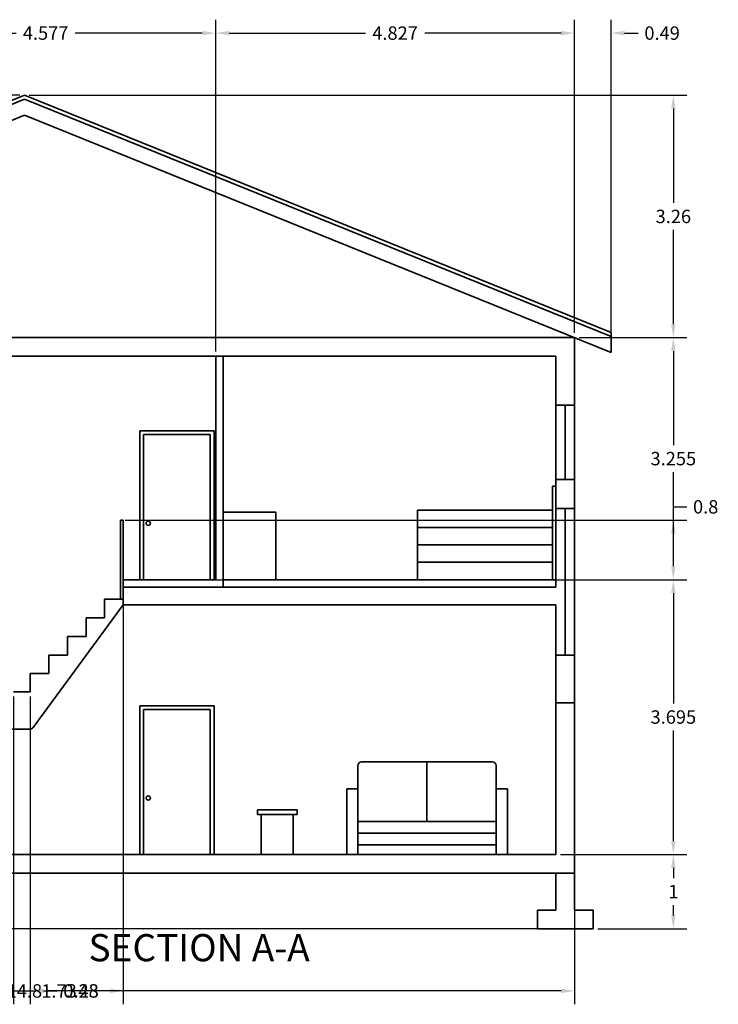
# Model space of a CAD drawing. Units: metres. Extents: x 14054 to 28215, y 4175 to 8383.
# Tile 6 of 6: x 14106.56 to 14115.96, y 4179.48 to 4192.72. Entities that reach past the tile are written whole.
import ezdxf

# ---------------------------------------------------------------- set-up
doc = ezdxf.new("R2010")
doc.units = ezdxf.units.M
for name, color, linetype, lineweight in [('A-ANNO-DIMS', 2, 'Continuous', 18), ('A-ANNO-NPLT', 9, 'Continuous', 13), ('A-ANNO-TEXT', 3, 'Continuous', 18), ('A-SECT', 1, 'Continuous', 35)]:
    doc.layers.add(name, color=color, linetype=linetype, lineweight=lineweight)
doc.styles.get("Standard").update_dxf_attribs({"font": 'arial.ttf'})
doc.dimstyles.get("Standard").update_dxf_attribs({"dimtxt": 0.18, "dimasz": 0.18, "dimexe": 0.18, "dimexo": 0.0625, "dimgap": 0.09, "dimtad": 0, "dimtih": 1, "dimtoh": 1, "dimdec": 4, "dimzin": 0, "dimdsep": 46, "dimtxsty": 'Standard', "dimcen": 0.09, "dimadec": 0, "dimazin": 0, "dimtfac": 1, "dimtdec": 4, "dimtofl": 0, "dimtmove": 0, "dimatfit": 3, "dimfxl": 1, "dimtolj": 1, "dimtzin": 0, "dimarcsym": 0})

# ---------------------------------------------------------------- blocks, each defined once
blk = doc.blocks.new('*D31')
at = {"layer": 'A-ANNO-DIMS', "color": 0, "lineweight": -2, "transparency": 16777216}
for p, q in [((14104.618, 4188.257), (14104.618, 4192.719)), ((14109.195, 4188.257), (14109.195, 4192.719)), ((14104.798, 4192.539), (14106.509, 4192.539)), ((14109.015, 4192.539), (14107.304, 4192.539))]:
    blk.add_line(p, q, dxfattribs=at)
at = {"layer": 'A-ANNO-DIMS', "color": 0, "transparency": 16777216}
for points in [[(14104.798, 4192.569), (14104.798, 4192.509), (14104.618, 4192.539)], [(14109.015, 4192.569), (14109.015, 4192.509), (14109.195, 4192.539)]]:
    blk.add_solid(points, dxfattribs=at)
at = {"layer": 'Defpoints', "color": 0, "transparency": 16777216}
for p in [(14109.195, 4192.539), (14104.618, 4188.194), (14109.195, 4188.194)]:
    blk.add_point(p, dxfattribs=at)
at = {"layer": 'A-ANNO-DIMS', "color": 0, "transparency": 16777216, "insert": (14106.907, 4192.539), "char_height": 0.18, "attachment_point": 5}
blk.add_mtext('\\A1;4.577', dxfattribs=at)
blk = doc.blocks.new('*D32')
at = {"layer": 'A-ANNO-DIMS', "color": 0, "lineweight": -2, "transparency": 16777216}
for p, q in [((14109.195, 4188.257), (14109.195, 4192.719)), ((14114.022, 4188.507), (14114.022, 4192.719)), ((14109.375, 4192.539), (14111.211, 4192.539)), ((14113.842, 4192.539), (14112.006, 4192.539))]:
    blk.add_line(p, q, dxfattribs=at)
at = {"layer": 'A-ANNO-DIMS', "color": 0, "transparency": 16777216}
for points in [[(14109.375, 4192.569), (14109.375, 4192.509), (14109.195, 4192.539)], [(14113.842, 4192.569), (14113.842, 4192.509), (14114.022, 4192.539)]]:
    blk.add_solid(points, dxfattribs=at)
at = {"layer": 'Defpoints', "color": 0, "transparency": 16777216}
for p in [(14114.022, 4192.539), (14114.022, 4188.444), (14109.195, 4188.194)]:
    blk.add_point(p, dxfattribs=at)
at = {"layer": 'A-ANNO-DIMS', "color": 0, "transparency": 16777216, "insert": (14111.608, 4192.539), "char_height": 0.18, "attachment_point": 5}
blk.add_mtext('\\A1;4.827', dxfattribs=at)
blk = doc.blocks.new('*D33')
at = {"layer": 'A-ANNO-DIMS', "color": 0, "lineweight": -2, "transparency": 16777216}
for p, q in [((14114.022, 4188.507), (14114.022, 4192.719)), ((14114.516, 4188.307), (14114.516, 4192.719)), ((14113.842, 4192.539), (14113.662, 4192.539)), ((14114.696, 4192.539), (14114.876, 4192.539))]:
    blk.add_line(p, q, dxfattribs=at)
at = {"layer": 'A-ANNO-DIMS', "color": 0, "transparency": 16777216}
for points in [[(14113.842, 4192.569), (14113.842, 4192.509), (14114.022, 4192.539)], [(14114.696, 4192.569), (14114.696, 4192.509), (14114.516, 4192.539)]]:
    blk.add_solid(points, dxfattribs=at)
at = {"layer": 'Defpoints', "color": 0, "transparency": 16777216}
for p in [(14114.516, 4192.539), (14114.022, 4188.444), (14114.516, 4188.244)]:
    blk.add_point(p, dxfattribs=at)
at = {"layer": 'A-ANNO-DIMS', "color": 0, "transparency": 16777216, "insert": (14115.2, 4192.539), "char_height": 0.18, "attachment_point": 5}
blk.add_mtext('\\A1;0.49', dxfattribs=at)
blk = doc.blocks.new('*D34')
at = {"layer": 'A-ANNO-DIMS', "color": 0, "lineweight": -2, "transparency": 16777216}
for p, q in [((14099.222, 4181.182), (14099.222, 4179.479)), ((14114.022, 4181.182), (14114.022, 4179.479)), ((14099.402, 4179.659), (14106.306, 4179.659)), ((14113.842, 4179.659), (14106.937, 4179.659))]:
    blk.add_line(p, q, dxfattribs=at)
at = {"layer": 'A-ANNO-DIMS', "color": 0, "transparency": 16777216}
for points in [[(14099.402, 4179.689), (14099.402, 4179.629), (14099.222, 4179.659)], [(14113.842, 4179.689), (14113.842, 4179.629), (14114.022, 4179.659)]]:
    blk.add_solid(points, dxfattribs=at)
at = {"layer": 'Defpoints', "color": 0, "transparency": 16777216}
for p in [(14099.222, 4181.244), (14114.022, 4181.244), (14114.022, 4179.659)]:
    blk.add_point(p, dxfattribs=at)
at = {"layer": 'A-ANNO-DIMS', "color": 0, "transparency": 16777216, "insert": (14106.622, 4179.659), "char_height": 0.18, "attachment_point": 5}
blk.add_mtext('\\A1;14.8', dxfattribs=at)
blk = doc.blocks.new('*D35')
at = {"layer": 'A-ANNO-DIMS', "color": 0, "lineweight": -2, "transparency": 16777216}
for p, q in [((14113.834, 4181.494), (14115.531, 4181.494)), ((14115.351, 4181.314), (14115.351, 4181.174)), ((14115.351, 4180.674), (14115.351, 4180.814)), ((14114.334, 4180.494), (14115.531, 4180.494))]:
    blk.add_line(p, q, dxfattribs=at)
at = {"layer": 'A-ANNO-DIMS', "color": 0, "transparency": 16777216}
for points in [[(14115.321, 4181.314), (14115.381, 4181.314), (14115.351, 4181.494)], [(14115.321, 4180.674), (14115.381, 4180.674), (14115.351, 4180.494)]]:
    blk.add_solid(points, dxfattribs=at)
at = {"layer": 'Defpoints', "color": 0, "transparency": 16777216}
for p in [(14113.772, 4181.494), (14115.351, 4181.494), (14114.272, 4180.494)]:
    blk.add_point(p, dxfattribs=at)
at = {"layer": 'A-ANNO-DIMS', "color": 0, "transparency": 16777216, "insert": (14115.351, 4180.994), "char_height": 0.18, "attachment_point": 5}
blk.add_mtext('\\A1;1', dxfattribs=at)
blk = doc.blocks.new('*D36')
at = {"layer": 'A-ANNO-DIMS', "color": 0, "lineweight": -2, "transparency": 16777216}
for p, q in [((14113.834, 4185.189), (14115.531, 4185.189)), ((14115.351, 4185.009), (14115.351, 4183.524)), ((14115.351, 4181.674), (14115.351, 4183.16)), ((14113.834, 4181.494), (14115.531, 4181.494))]:
    blk.add_line(p, q, dxfattribs=at)
at = {"layer": 'A-ANNO-DIMS', "color": 0, "transparency": 16777216}
for points in [[(14115.321, 4185.009), (14115.381, 4185.009), (14115.351, 4185.189)], [(14115.321, 4181.674), (14115.381, 4181.674), (14115.351, 4181.494)]]:
    blk.add_solid(points, dxfattribs=at)
at = {"layer": 'Defpoints', "color": 0, "transparency": 16777216}
for p in [(14113.772, 4185.189), (14115.351, 4185.189), (14113.772, 4181.494)]:
    blk.add_point(p, dxfattribs=at)
at = {"layer": 'A-ANNO-DIMS', "color": 0, "transparency": 16777216, "insert": (14115.351, 4183.342), "char_height": 0.18, "attachment_point": 5}
blk.add_mtext('\\A1;3.695', dxfattribs=at)
blk = doc.blocks.new('*D37')
at = {"layer": 'A-ANNO-DIMS', "color": 0, "lineweight": -2, "transparency": 16777216}
for p, q in [((14114.084, 4188.444), (14115.531, 4188.444)), ((14115.351, 4188.264), (14115.351, 4186.999)), ((14115.351, 4185.369), (14115.351, 4186.635)), ((14113.834, 4185.189), (14115.531, 4185.189))]:
    blk.add_line(p, q, dxfattribs=at)
at = {"layer": 'A-ANNO-DIMS', "color": 0, "transparency": 16777216}
for points in [[(14115.321, 4188.264), (14115.381, 4188.264), (14115.351, 4188.444)], [(14115.321, 4185.369), (14115.381, 4185.369), (14115.351, 4185.189)]]:
    blk.add_solid(points, dxfattribs=at)
at = {"layer": 'Defpoints', "color": 0, "transparency": 16777216}
for p in [(14114.022, 4188.444), (14115.351, 4188.444), (14113.772, 4185.189)]:
    blk.add_point(p, dxfattribs=at)
at = {"layer": 'A-ANNO-DIMS', "color": 0, "transparency": 16777216, "insert": (14115.351, 4186.817), "char_height": 0.18, "attachment_point": 5}
blk.add_mtext('\\A1;3.255', dxfattribs=at)
blk = doc.blocks.new('*D38')
at = {"layer": 'A-ANNO-DIMS', "color": 0, "lineweight": -2, "transparency": 16777216}
for p, q in [((14106.684, 4191.704), (14115.531, 4191.704)), ((14115.351, 4191.524), (14115.351, 4190.256)), ((14115.351, 4188.624), (14115.351, 4189.892)), ((14114.084, 4188.444), (14115.531, 4188.444))]:
    blk.add_line(p, q, dxfattribs=at)
at = {"layer": 'A-ANNO-DIMS', "color": 0, "transparency": 16777216}
for points in [[(14115.321, 4191.524), (14115.381, 4191.524), (14115.351, 4191.704)], [(14115.321, 4188.624), (14115.381, 4188.624), (14115.351, 4188.444)]]:
    blk.add_solid(points, dxfattribs=at)
at = {"layer": 'Defpoints', "color": 0, "transparency": 16777216}
for p in [(14106.622, 4191.704), (14115.351, 4191.704), (14114.022, 4188.444)]:
    blk.add_point(p, dxfattribs=at)
at = {"layer": 'A-ANNO-DIMS', "color": 0, "transparency": 16777216, "insert": (14115.351, 4190.074), "char_height": 0.18, "attachment_point": 5}
blk.add_mtext('\\A1;3.26', dxfattribs=at)
blk = doc.blocks.new('*D39')
at = {"layer": 'A-ANNO-DIMS', "color": 0, "lineweight": -2, "transparency": 16777216}
for p, q in [((14106.559, 4191.704), (14097.707, 4191.704)), ((14097.887, 4191.524), (14097.887, 4186.28)), ((14097.887, 4180.674), (14097.887, 4185.919)), ((14114.209, 4180.494), (14097.707, 4180.494))]:
    blk.add_line(p, q, dxfattribs=at)
at = {"layer": 'A-ANNO-DIMS', "color": 0, "transparency": 16777216}
for points in [[(14097.857, 4191.524), (14097.917, 4191.524), (14097.887, 4191.704)], [(14097.857, 4180.674), (14097.917, 4180.674), (14097.887, 4180.494)]]:
    blk.add_solid(points, dxfattribs=at)
at = {"layer": 'Defpoints', "color": 0, "transparency": 16777216}
for p in [(14097.887, 4191.704), (14106.622, 4191.704), (14114.272, 4180.494)]:
    blk.add_point(p, dxfattribs=at)
at = {"layer": 'A-ANNO-DIMS', "color": 0, "transparency": 16777216, "insert": (14097.887, 4186.099), "char_height": 0.18, "attachment_point": 5}
blk.add_mtext('\\A1;11.21', dxfattribs=at)
blk = doc.blocks.new('*D60')
at = {"layer": 'A-ANNO-DIMS', "color": 0, "lineweight": -2, "transparency": 16777216}
for p, q in [((14107.951, 4184.863), (14107.951, 4179.479)), ((14106.224, 4183.368), (14106.224, 4179.479)), ((14106.404, 4179.659), (14106.772, 4179.659)), ((14107.771, 4179.659), (14107.403, 4179.659))]:
    blk.add_line(p, q, dxfattribs=at)
at = {"layer": 'A-ANNO-DIMS', "color": 0, "transparency": 16777216}
for points in [[(14106.404, 4179.689), (14106.404, 4179.629), (14106.224, 4179.659)], [(14107.771, 4179.689), (14107.771, 4179.629), (14107.951, 4179.659)]]:
    blk.add_solid(points, dxfattribs=at)
at = {"layer": 'Defpoints', "color": 0, "transparency": 16777216}
for p in [(14107.951, 4184.925), (14106.224, 4183.431), (14107.951, 4179.659)]:
    blk.add_point(p, dxfattribs=at)
at = {"layer": 'A-ANNO-DIMS', "color": 0, "transparency": 16777216, "insert": (14107.088, 4179.659), "char_height": 0.18, "attachment_point": 5}
blk.add_mtext('\\A1;1.73', dxfattribs=at)
blk = doc.blocks.new('*D62')
at = {"layer": 'A-ANNO-DIMS', "color": 0, "lineweight": -2, "transparency": 16777216}
for p, q in [((14106.473765, 4183.618165), (14106.473765, 4179.479065)), ((14106.701342, 4183.618165), (14106.701342, 4179.479065)), ((14106.293765, 4179.659065), (14106.113765, 4179.659065)), ((14106.881342, 4179.659065), (14107.061342, 4179.659065))]:
    blk.add_line(p, q, dxfattribs=at)
at = {"layer": 'A-ANNO-DIMS', "color": 0, "transparency": 16777216}
for points in [[(14106.293765, 4179.689065), (14106.293765, 4179.629065), (14106.473765, 4179.659065)], [(14106.881342, 4179.689065), (14106.881342, 4179.629065), (14106.701342, 4179.659065)]]:
    blk.add_solid(points, dxfattribs=at)
at = {"layer": 'Defpoints', "color": 0, "transparency": 16777216}
for p in [(14106.473765, 4183.680665), (14106.701342, 4183.680665), (14106.701342, 4179.659065)]:
    blk.add_point(p, dxfattribs=at)
at = {"layer": 'A-ANNO-DIMS', "color": 0, "transparency": 16777216, "insert": (14107.385121, 4179.659065), "char_height": 0.18, "attachment_point": 5}
blk.add_mtext('\\A1;0.23', dxfattribs=at)
blk = doc.blocks.new('*D63')
at = {"layer": 'A-ANNO-DIMS', "color": 0, "lineweight": -2, "transparency": 16777216}
for p, q in [((14106.224, 4183.118), (14106.224, 4179.479)), ((14106.7, 4183.118), (14106.7, 4179.479)), ((14106.044, 4179.659), (14105.864, 4179.659)), ((14106.88, 4179.659), (14107.06, 4179.659))]:
    blk.add_line(p, q, dxfattribs=at)
at = {"layer": 'A-ANNO-DIMS', "color": 0, "transparency": 16777216}
for points in [[(14106.044, 4179.689), (14106.044, 4179.629), (14106.224, 4179.659)], [(14106.88, 4179.689), (14106.88, 4179.629), (14106.7, 4179.659)]]:
    blk.add_solid(points, dxfattribs=at)
at = {"layer": 'Defpoints', "color": 0, "transparency": 16777216}
for p in [(14106.224, 4183.181), (14106.7, 4183.181), (14106.7, 4179.659)]:
    blk.add_point(p, dxfattribs=at)
at = {"layer": 'A-ANNO-DIMS', "color": 0, "transparency": 16777216, "insert": (14107.383, 4179.659), "char_height": 0.18, "attachment_point": 5}
blk.add_mtext('\\A1;0.48', dxfattribs=at)
blk = doc.blocks.new('*D66')
at = {"layer": 'A-ANNO-DIMS', "color": 0, "lineweight": -2, "transparency": 16777216}
for p, q in [((14115.351, 4185.989), (14115.351, 4186.169)), ((14115.351, 4186.169), (14115.531, 4186.169)), ((14107.975, 4185.989), (14115.531, 4185.989)), ((14115.351, 4185.369), (14115.351, 4185.809)), ((14108.014, 4185.189), (14115.531, 4185.189))]:
    blk.add_line(p, q, dxfattribs=at)
at = {"layer": 'A-ANNO-DIMS', "color": 0, "transparency": 16777216}
for points in [[(14115.321, 4185.809), (14115.381, 4185.809), (14115.351, 4185.989)], [(14115.321, 4185.369), (14115.381, 4185.369), (14115.351, 4185.189)]]:
    blk.add_solid(points, dxfattribs=at)
at = {"layer": 'Defpoints', "color": 0, "transparency": 16777216}
for p in [(14107.913, 4185.989), (14115.351, 4185.989), (14107.951, 4185.189)]:
    blk.add_point(p, dxfattribs=at)
at = {"layer": 'A-ANNO-DIMS', "color": 0, "transparency": 16777216, "insert": (14115.786, 4186.169), "char_height": 0.18, "attachment_point": 5}
blk.add_mtext('\\A1;0.8', dxfattribs=at)

msp = doc.modelspace()

# ---------------------------------------------------------------- linework, layer by layer
at = {"layer": 'A-ANNO-NPLT'}
for p in [(14112.2507, 4185.8914), (14112.2507, 4185.6573), (14112.2507, 4185.4232), (14109.245, 4181.4941)]:
    msp.add_point(p, dxfattribs=at)
at = {"layer": 'A-SECT'}
for p, q in [((14098.7216, 4188.511), (14106.6216, 4191.7043)), ((14098.7216, 4188.4571), (14106.6216, 4191.6503)), ((14106.6216, 4191.7043), (14114.5165, 4188.5137)), ((14106.6216, 4191.6503), (14114.5165, 4188.4598)), ((14098.7216, 4188.2414), (14106.6216, 4191.4346)), ((14106.6216, 4191.4346), (14114.5165, 4188.2441)), ((14099.2216, 4188.4441), (14114.0216, 4188.4441)), ((14109.195, 4188.4441), (14109.295, 4188.4441)), ((14114.0216, 4188.4441), (14114.0216, 4181.2441)), ((14114.5165, 4188.2441), (14114.5165, 4188.5137)), ((14099.4716, 4188.1941), (14113.7716, 4188.1941)), ((14109.195, 4185.1891), (14109.195, 4188.1941)), ((14109.295, 4185.0891), (14109.295, 4188.1941)), ((14113.7716, 4188.1941), (14113.7716, 4185.0891)), ((14113.7716, 4187.5366), (14114.0216, 4187.5366)), ((14113.8966, 4187.5366), (14113.8966, 4186.5366)), ((14109.1723, 4187.1895), (14108.1723, 4187.1895)), ((14108.1723, 4187.1895), (14108.1723, 4185.1891)), ((14109.1223, 4187.1395), (14108.2223, 4187.1395)), ((14108.2223, 4187.1395), (14108.2223, 4185.1891)), ((14109.1223, 4185.1891), (14109.1223, 4187.1395)), ((14109.1723, 4185.1891), (14109.1723, 4187.1895)), ((14113.724, 4185.1891), (14113.724, 4186.4482)), ((14113.724, 4186.4482), (14113.7716, 4186.4482)), ((14113.7716, 4186.5366), (14114.0216, 4186.5366)), ((14109.295, 4186.0972), (14110.0021, 4186.0972)), ((14110.0021, 4186.0972), (14110.0021, 4185.1891)), ((14111.9084, 4185.1891), (14111.9084, 4186.1255)), ((14111.9084, 4186.1255), (14113.724, 4186.1255)), ((14113.7716, 4186.1467), (14114.0216, 4186.1467)), ((14113.8966, 4186.1467), (14113.8966, 4184.1738)), ((14107.9513, 4185.9891), (14107.9128, 4185.9891)), ((14107.9128, 4185.9891), (14107.9128, 4184.9253)), ((14107.9513, 4185.1891), (14107.9513, 4185.9891)), ((14111.9084, 4185.8914), (14113.724, 4185.8914)), ((14111.9084, 4185.6573), (14113.724, 4185.6573)), ((14111.9084, 4185.4232), (14113.724, 4185.4232)), ((14107.9513, 4185.1891), (14109.195, 4185.1891)), ((14107.9513, 4185.1891), (14107.9513, 4184.8491)), ((14109.295, 4185.1891), (14113.7716, 4185.1891)), ((14107.9513, 4185.0891), (14113.7716, 4185.0891)), ((14107.9513, 4184.8491), (14106.7398, 4183.201)), ((14107.9513, 4184.9253), (14107.7013, 4184.9253)), ((14107.7013, 4184.9253), (14107.7013, 4184.6753)), ((14113.7716, 4184.8491), (14107.9513, 4184.8491)), ((14113.7716, 4184.8491), (14113.7716, 4181.4941)), ((14107.7013, 4184.6753), (14107.4513, 4184.6753)), ((14107.4513, 4184.6753), (14107.4513, 4184.4253)), ((14107.4513, 4184.4253), (14107.2013, 4184.4253)), ((14107.2013, 4184.4253), (14107.2013, 4184.1753)), ((14107.2013, 4184.1753), (14106.9513, 4184.1753)), ((14106.9513, 4184.1753), (14106.9513, 4183.9253)), ((14113.7716, 4184.1738), (14114.0216, 4184.1738)), ((14106.9513, 4183.9253), (14106.7013, 4183.9253)), ((14106.7013, 4183.9253), (14106.7013, 4183.6807)), ((14106.7013, 4183.6807), (14106.4738, 4183.6807)), ((14113.7716, 4183.5311), (14114.0216, 4183.5311)), ((14109.1723, 4183.4945), (14108.1723, 4183.4945)), ((14108.1723, 4183.4945), (14108.1723, 4181.4941)), ((14109.1223, 4183.4445), (14108.2223, 4183.4445)), ((14108.2223, 4183.4445), (14108.2223, 4181.4941)), ((14109.1223, 4181.4941), (14109.1223, 4183.4445)), ((14109.1723, 4181.4941), (14109.1723, 4183.4945)), ((14106.2238, 4183.1807), (14106.6995, 4183.1807)), ((14112.0372, 4182.7396), (14111.1585, 4182.7396)), ((14112.0372, 4181.9358), (14112.0372, 4182.7396)), ((14112.0372, 4182.7396), (14112.916, 4182.7396)), ((14111.1085, 4182.3776), (14111.1085, 4182.6896)), ((14112.966, 4182.3776), (14112.966, 4182.6896)), ((14110.9594, 4181.4941), (14110.9594, 4182.3776)), ((14110.9594, 4182.3776), (14111.1085, 4182.3776)), ((14111.1085, 4182.3776), (14111.1085, 4181.4941)), ((14113.1186, 4182.3776), (14112.966, 4182.3776)), ((14112.966, 4182.3776), (14112.966, 4181.4941)), ((14113.1186, 4181.4941), (14113.1186, 4182.3776)), ((14109.7555, 4182.0962), (14110.2901, 4182.0962)), ((14109.7555, 4182.0962), (14109.7555, 4182.0318)), ((14110.2901, 4182.0318), (14110.2901, 4182.0962)), ((14109.7555, 4182.0318), (14110.2901, 4182.0318)), ((14109.8067, 4181.4941), (14109.8067, 4182.0318)), ((14110.2389, 4182.0318), (14110.2389, 4181.4941)), ((14111.1085, 4181.9358), (14112.966, 4181.9358)), ((14111.1085, 4181.7801), (14112.966, 4181.7801)), ((14111.1085, 4181.6236), (14112.966, 4181.6236)), ((14099.4716, 4181.4941), (14113.7716, 4181.4941)), ((14099.2216, 4181.2441), (14114.0216, 4181.2441)), ((14113.7716, 4181.2441), (14113.7716, 4180.7441)), ((14114.0216, 4181.2441), (14114.0216, 4180.7441)), ((14113.7716, 4180.7441), (14113.5216, 4180.7441)), ((14113.5216, 4180.7441), (14113.5216, 4180.4941)), ((14114.0216, 4180.7441), (14114.2716, 4180.7441)), ((14114.2716, 4180.7441), (14114.2716, 4180.4941)), ((14113.5216, 4180.4941), (14114.2716, 4180.4941))]:
    msp.add_line(p, q, dxfattribs=at)
for centre in [(14108.2879, 4185.9485), (14108.2879, 4182.2535)]:
    msp.add_circle(centre, 0.0289, dxfattribs=at)
for centre, start, end in [((14106.6995, 4183.2307), 270, 323.67833), ((14111.1585, 4182.6896), 90, 180), ((14112.916, 4182.6896), 0, 90)]:
    msp.add_arc(centre, 0.05, start, end, dxfattribs=at)

# ---------------------------------------------------------------- texts
at = {"layer": 'A-ANNO-TEXT'}
msp.add_text('SECTION A-A', height=0.365459, dxfattribs=at).set_placement((14107.4846, 4180.058))

# ---------------------------------------------------------------- dimensions: what is measured, and where the dimension line sits
at = {"layer": 'A-ANNO-DIMS'}
for base, p1, p2, override, picture, middle in [((14109.195, 4192.5393), (14104.6184, 4188.1941), (14109.195, 4188.1941), {"dimdec": 3, "dimlfac": 1, "dimrnd": 0, "dimzin": 0, "dimdsep": 46, "dimlunit": 2}, '*D31', (14106.9067, 4192.5393)), ((14114.0216, 4192.5393), (14109.195, 4188.1941), (14114.0216, 4188.4441), {"dimdec": 3, "dimlfac": 1, "dimrnd": 0, "dimzin": 0, "dimdsep": 46, "dimlunit": 2}, '*D32', (14111.6083, 4192.5393)), ((14114.5165, 4192.5393), (14114.0216, 4188.4441), (14114.5165, 4188.2441), {"dimdec": 2, "dimlfac": 1, "dimrnd": 0, "dimzin": 0, "dimdsep": 46, "dimlunit": 2}, '*D33', (14115.2004, 4192.5393)), ((14107.9513, 4179.6591), (14106.2238, 4183.4307), (14107.9513, 4184.9253), {"dimdec": 2, "dimlfac": 1, "dimrnd": 0, "dimzin": 0, "dimdsep": 46, "dimlunit": 2}, '*D60', (14107.0876, 4179.6591)), ((14106.7013, 4179.6591), (14106.4738, 4183.6807), (14106.7013, 4183.6807), {"dimdec": 2, "dimlfac": 1, "dimrnd": 0, "dimzin": 0, "dimdsep": 46, "dimlunit": 2}, '*D62', (14107.3851, 4179.6591)), ((14106.6995, 4179.6591), (14106.2238, 4183.1807), (14106.6995, 4183.1807), {"dimdec": 2, "dimlfac": 1, "dimrnd": 0, "dimzin": 0, "dimdsep": 46, "dimlunit": 2}, '*D63', (14107.3835, 4179.6591)), ((14114.0216, 4179.6591), (14099.2216, 4181.2441), (14114.0216, 4181.2441), {"dimdec": 1, "dimlfac": 1, "dimrnd": 0, "dimzin": 0, "dimdsep": 46, "dimlunit": 2}, '*D34', (14106.6216, 4179.6591))]:
    dim = msp.add_linear_dim(base=base, p1=p1, p2=p2, dimstyle='Standard', override=override, dxfattribs=at)
    dim.commit()
    dim.dimension.update_dxf_attribs({"geometry": picture, "text_midpoint": middle})
for base, p1, p2, override, picture, middle in [((14097.8866, 4191.7043), (14114.2716, 4180.4941), (14106.6216, 4191.7043), {"dimdec": 2, "dimlfac": 1, "dimrnd": 0, "dimzin": 0, "dimdsep": 46, "dimlunit": 2}, '*D39', (14097.8866, 4186.0992)), ((14115.3515, 4191.7043), (14114.0216, 4188.4441), (14106.6216, 4191.7043), {"dimdec": 2, "dimlfac": 1, "dimrnd": 0, "dimzin": 0, "dimdsep": 46, "dimlunit": 2}, '*D38', (14115.3515, 4190.0742)), ((14115.3515, 4188.4441), (14113.7716, 4185.1891), (14114.0216, 4188.4441), {"dimdec": 3, "dimlfac": 1, "dimrnd": 0, "dimzin": 0, "dimdsep": 46, "dimlunit": 2}, '*D37', (14115.3515, 4186.8166)), ((14115.3515, 4185.9891), (14107.9513, 4185.1891), (14107.9128, 4185.9891), {"dimdec": 1, "dimlfac": 1, "dimrnd": 0, "dimzin": 0, "dimdsep": 46, "dimlunit": 2}, '*D66', (14115.7855, 4186.1691)), ((14115.3515, 4185.1891), (14113.7716, 4181.4941), (14113.7716, 4185.1891), {"dimdec": 3, "dimlfac": 1, "dimrnd": 0, "dimzin": 0, "dimdsep": 46, "dimlunit": 2}, '*D36', (14115.3515, 4183.3416)), ((14115.3515, 4181.4941), (14114.2716, 4180.4941), (14113.7716, 4181.4941), {"dimdec": 0, "dimlfac": 1, "dimrnd": 0, "dimzin": 0, "dimdsep": 46, "dimlunit": 2}, '*D35', (14115.3515, 4180.9941))]:
    dim = msp.add_linear_dim(base=base, p1=p1, p2=p2, angle=90, dimstyle='Standard', override=override, dxfattribs=at)
    dim.commit()
    dim.dimension.update_dxf_attribs({"geometry": picture, "text_midpoint": middle})

doc.saveas('drawing.dxf')
